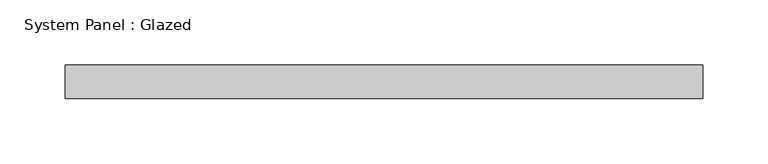
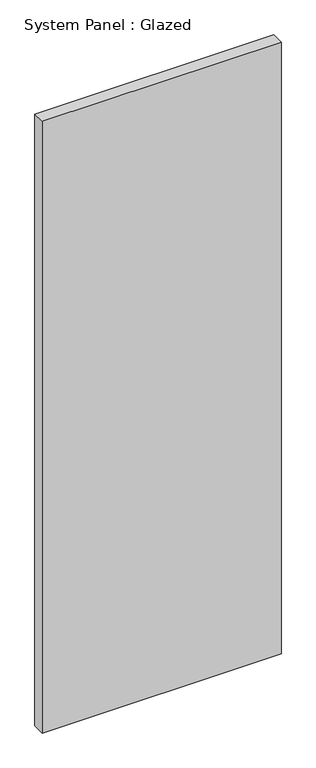
"""IFC4 building model written with IfcOpenShell, lengths in millimetres: plate geometry, System Panel : Glazed."""

from ifc_helpers import new_model, si_unit, origin, origin_with_axes, place, context, project, spatial, polyline, outline, extrude, source, transform, mapped, element, save


def system_panel_glazed_a3f5704d(model_context):
    return source(origin(), model_context, "Body", "SweptSolid", [
        extrude(outline(polyline([(243.7299185, 19.05), (-243.7299185, 19.05), (-243.7299185, 44.45), (243.7299185, 44.45), (243.7299185, 19.05)])), origin_with_axes(), (0.0, 0.0, 1.0), 1319.9815053),
    ])


if __name__ == "__main__":
    model = new_model("IFC4")
    model_context = context("Model", 3, world=origin())
    ifc_project = project(units=[si_unit("LENGTHUNIT", "METRE", prefix="MILLI")], contexts=[model_context])
    site = spatial("IfcSite", under=ifc_project)
    building = spatial("IfcBuilding", under=site)
    placement = place(None, origin())
    system_panel_glazed_shape = system_panel_glazed_a3f5704d(model_context)
    element("IfcPlate", 1, ObjectType="System Panel : Glazed", at=placement, inside=building, context=model_context, shape_type="MappedRepresentation", body=[
        mapped(system_panel_glazed_shape, transform((0.0, 0.0, 0.0), x_axis=(1.0, 0.0, 0.0), y_axis=(0.0, 1.0, 0.0), z_axis=(0.0, 0.0, 1.0))),
    ])
    save(model, "model.ifc")

# Revit data of these elements
# Type "System Panel : Glazed"
#   Construction Type Id = "GSP4R"
#   Analytic Construction = "1/8 in Pilkington single glazing"
#   Visual Light Transmittance = 0.9
#   Solar Heat Gain Coefficient = 0.86
#   Heat Transfer Coefficient (U) = 1.18115 BTU/(h·ft²·°F)
#   Define Thermal Properties by = 1
# Element 1 (IfcPlate, "System Panel : Glazed")
#   Materials on its faces: "Glass"
# Materials
#   "Glass": class "Glass", colour RGB 0 128 192, transparency 0.75, Description = "Soda Lime Glass", Cost = 0
